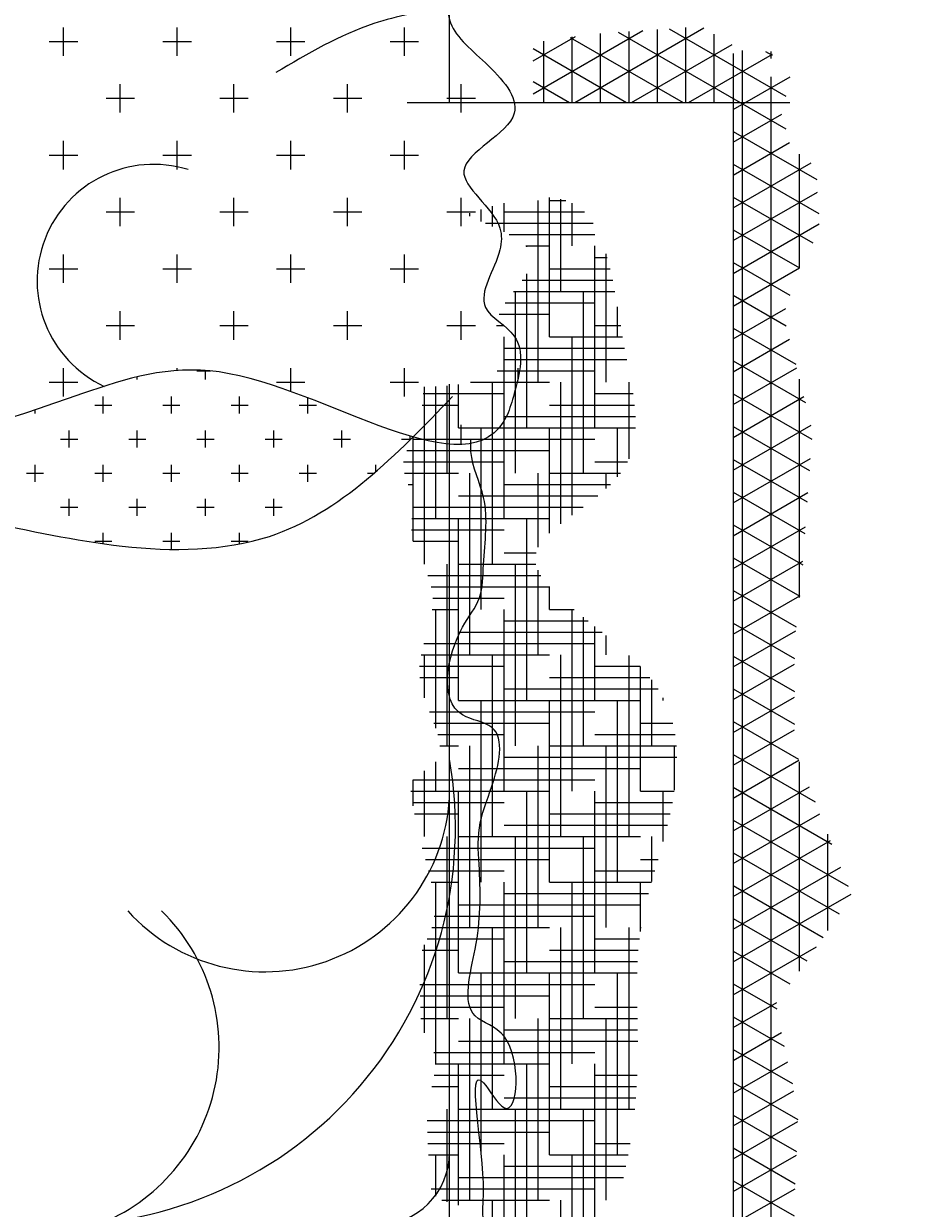
# Model space of a CAD drawing. Units: inches. Extents: x 2330 to 3943, y 1763 to 3461.
# Tile 18 of 40: x 3179 to 3231, y 2593 to 2662. Entities that reach past the tile are written whole.
import ezdxf

# ---------------------------------------------------------------- set-up
doc = ezdxf.new("R2010")
doc.units = ezdxf.units.IN
doc.layers.add('A-ANNO-DIMS', color=2, linetype='Continuous', lineweight=18)
doc.layers.add('A-FURN', color=8, linetype='Continuous', lineweight=13)
doc.styles.get("Standard").update_dxf_attribs({"font": 'arial.ttf'})
doc.dimstyles.get("Standard").update_dxf_attribs({"dimtxt": 0.18, "dimasz": 0.18, "dimexe": 0.18, "dimexo": 0.0625, "dimgap": 0.09, "dimtad": 0, "dimtih": 1, "dimtoh": 1, "dimdec": 4, "dimzin": 0, "dimdsep": 46, "dimtxsty": 'Standard', "dimcen": 0.09, "dimadec": 0, "dimazin": 0, "dimtfac": 1, "dimtdec": 4, "dimtofl": 0, "dimtmove": 0, "dimatfit": 3, "dimfxl": 1, "dimtolj": 1, "dimtzin": 0, "dimarcsym": 0})

# ---------------------------------------------------------------- blocks, each defined once
blk = doc.blocks.new('A$C200C7901')
for p, q in [((2, 1.6055), (2, 2.3334)), ((2.3121, 1.6596), (2.3121, 0.0201)), ((1.9533, 1.6055), (2.3741, 1.6055)), ((1.9533, 1.6055), (2.3741, 1.6055)), ((2, 0.2957), (2, 1.2957)), ((2.0224, 0.9977), (2.0224, 1.1977)), ((2.0224, 0.9977), (2.0224, 1.1977)), ((1.9974, 0.5977), (1.9974, 0.7977)), ((1.9974, 0.5977), (1.9974, 0.7977)), ((2.0724, 0.5977), (2.0724, 0.7977)), ((2.0724, 0.5977), (2.0724, 0.7977)), ((2.1474, 0.5977), (2.1474, 0.7977)), ((2.1474, 0.5977), (2.1474, 0.7977)), ((1.9849, 0.5477), (1.9849, 0.7477)), ((1.9849, 0.5477), (1.9849, 0.7477)), ((2.0599, 0.5477), (2.0599, 0.7477)), ((2.0599, 0.5477), (2.0599, 0.7477)), ((2.1349, 0.5477), (2.1349, 0.7477)), ((2.1349, 0.5477), (2.1349, 0.7477))]:
    blk.add_line(p, q)
at = {"linetype": 'ByBlock'}
for p, q in [((1.5754, 1.657), (1.5754, 1.6883)), ((1.5754, 1.657), (1.5754, 1.6883)), ((1.7004, 1.657), (1.7004, 1.6883)), ((1.7004, 1.657), (1.7004, 1.6883)), ((1.8254, 1.657), (1.8254, 1.6883)), ((1.8254, 1.657), (1.8254, 1.6883)), ((1.9504, 1.657), (1.9504, 1.6883)), ((1.9504, 1.657), (1.9504, 1.6883)), ((2.0919, 1.6152), (2.2125, 1.6848)), ((2.0919, 1.6152), (2.2125, 1.6848)), ((2.1377, 1.6055), (2.2798, 1.6876)), ((2.1377, 1.6055), (2.2798, 1.6876)), ((2.1662, 1.6055), (2.1662, 1.6817)), ((2.1662, 1.6055), (2.1662, 1.6817)), ((2.1854, 1.683), (2.3697, 1.5766)), ((2.1854, 1.683), (2.3697, 1.5766)), ((2.1974, 1.6055), (2.1974, 1.6838)), ((2.1974, 1.6055), (2.1974, 1.6838)), ((2.2287, 1.6055), (2.2287, 1.6859)), ((2.2287, 1.6055), (2.2287, 1.6859)), ((2.2414, 1.6868), (2.3699, 1.6126)), ((2.2414, 1.6868), (2.3699, 1.6126)), ((2.2599, 1.6055), (2.2599, 1.688)), ((2.2599, 1.6055), (2.2599, 1.688)), ((1.5597, 1.6727), (1.591, 1.6727)), ((1.5597, 1.6727), (1.591, 1.6727)), ((1.6847, 1.6727), (1.716, 1.6727)), ((1.6847, 1.6727), (1.716, 1.6727)), ((1.8097, 1.6727), (1.841, 1.6727)), ((1.8097, 1.6727), (1.841, 1.6727)), ((1.9347, 1.6727), (1.966, 1.6727)), ((1.9347, 1.6727), (1.966, 1.6727)), ((2.0919, 1.6513), (2.1386, 1.6782)), ((2.0919, 1.6513), (2.1386, 1.6782)), ((2.1037, 1.6055), (2.1037, 1.673)), ((2.1037, 1.6055), (2.1037, 1.673)), ((2.1327, 1.6773), (2.2571, 1.6055)), ((2.1327, 1.6773), (2.2571, 1.6055)), ((2.1349, 1.6055), (2.1349, 1.6777)), ((2.1349, 1.6055), (2.1349, 1.6777)), ((2.2002, 1.6055), (2.3109, 1.6694)), ((2.2002, 1.6055), (2.3109, 1.6694)), ((2.2912, 1.6055), (2.2912, 1.6809)), ((2.2912, 1.6055), (2.2912, 1.6809)), ((2.0919, 1.6649), (2.1946, 1.6055)), ((2.0919, 1.6649), (2.1946, 1.6055)), ((2.2627, 1.6055), (2.3551, 1.6589)), ((2.2627, 1.6055), (2.3551, 1.6589)), ((2.3224, 0.0468), (2.3224, 1.6627)), ((2.3224, 0.0468), (2.3224, 1.6627)), ((2.3476, 1.6616), (2.3547, 1.6575)), ((2.3476, 1.6616), (2.3547, 1.6575)), ((2.3537, 1.6539), (2.3537, 1.6616)), ((2.3537, 1.6539), (2.3537, 1.6616)), ((2.3121, 1.598), (2.3745, 1.634)), ((2.3121, 1.598), (2.3745, 1.634)), ((2.3537, 0.0056), (2.3537, 1.634)), ((2.3537, 0.0056), (2.3537, 1.634)), ((1.6379, 1.5945), (1.6379, 1.6258)), ((1.6379, 1.5945), (1.6379, 1.6258)), ((1.7629, 1.5945), (1.7629, 1.6258)), ((1.7629, 1.5945), (1.7629, 1.6258)), ((1.8879, 1.5945), (1.8879, 1.6258)), ((1.8879, 1.5945), (1.8879, 1.6258)), ((2.0129, 1.5945), (2.0129, 1.6258)), ((2.0129, 1.5945), (2.0129, 1.6258)), ((2.0919, 1.6288), (2.1321, 1.6055)), ((2.0919, 1.6288), (2.1321, 1.6055)), ((1.6222, 1.6102), (1.6535, 1.6102)), ((1.6222, 1.6102), (1.6535, 1.6102)), ((1.7472, 1.6102), (1.7785, 1.6102)), ((1.7472, 1.6102), (1.7785, 1.6102)), ((1.8722, 1.6102), (1.9035, 1.6102)), ((1.8722, 1.6102), (1.9035, 1.6102)), ((1.9972, 1.6102), (2.0285, 1.6102)), ((1.9972, 1.6102), (2.0285, 1.6102)), ((2.3121, 1.5619), (2.3654, 1.5926)), ((2.3121, 1.5619), (2.3654, 1.5926)), ((2.3121, 1.5738), (2.404, 1.5208)), ((2.3121, 1.5738), (2.404, 1.5208)), ((1.5754, 1.532), (1.5754, 1.5633)), ((1.5754, 1.532), (1.5754, 1.5633)), ((1.7004, 1.532), (1.7004, 1.5633)), ((1.7004, 1.532), (1.7004, 1.5633)), ((1.8254, 1.532), (1.8254, 1.5633)), ((1.8254, 1.532), (1.8254, 1.5633)), ((1.9504, 1.532), (1.9504, 1.5633)), ((1.9504, 1.532), (1.9504, 1.5633)), ((2.3121, 1.5258), (2.3739, 1.5615)), ((2.3121, 1.5258), (2.3739, 1.5615)), ((1.5597, 1.5477), (1.591, 1.5477)), ((1.5597, 1.5477), (1.591, 1.5477)), ((1.6847, 1.5477), (1.716, 1.5477)), ((1.6847, 1.5477), (1.716, 1.5477)), ((1.8097, 1.5477), (1.841, 1.5477)), ((1.8097, 1.5477), (1.841, 1.5477)), ((1.9347, 1.5477), (1.966, 1.5477)), ((1.9347, 1.5477), (1.966, 1.5477)), ((2.3121, 1.4897), (2.3979, 1.5393)), ((2.3121, 1.4897), (2.3979, 1.5393)), ((2.3849, 1.4236), (2.3849, 1.5486)), ((2.3849, 1.4236), (2.3849, 1.5486)), ((2.3121, 1.5377), (2.406, 1.4835)), ((2.3121, 1.5377), (2.406, 1.4835)), ((1.6379, 1.4695), (1.6379, 1.5008)), ((1.6379, 1.4695), (1.6379, 1.5008)), ((1.7629, 1.4695), (1.7629, 1.5008)), ((1.7629, 1.4695), (1.7629, 1.5008)), ((1.8879, 1.4695), (1.8879, 1.5008)), ((1.8879, 1.4695), (1.8879, 1.5008)), ((2.0129, 1.4695), (2.0129, 1.5008)), ((2.0129, 1.4695), (2.0129, 1.5008)), ((2.1099, 1.3477), (2.1099, 1.5009)), ((2.1099, 1.3477), (2.1099, 1.5009)), ((2.1224, 1.3977), (2.1224, 1.4992)), ((2.1224, 1.3977), (2.1224, 1.4992)), ((2.3121, 1.4537), (2.4047, 1.5071)), ((2.3121, 1.4537), (2.4047, 1.5071)), ((2.3121, 1.5016), (2.3997, 1.4511)), ((2.3121, 1.5016), (2.3997, 1.4511)), ((2.0349, 1.4748), (2.0349, 1.4879)), ((2.0349, 1.4748), (2.0349, 1.4879)), ((2.0474, 1.4691), (2.0474, 1.4915)), ((2.0474, 1.4691), (2.0474, 1.4915)), ((2.0599, 1.4631), (2.0599, 1.4948)), ((2.0599, 1.4631), (2.0599, 1.4948)), ((2.0974, 1.2977), (2.0974, 1.4977)), ((2.0974, 1.2977), (2.0974, 1.4977)), ((2.1099, 1.4977), (2.1279, 1.4977)), ((2.1099, 1.4977), (2.1279, 1.4977)), ((2.1349, 1.4477), (2.1349, 1.4949)), ((2.1349, 1.4477), (2.1349, 1.4949)), ((1.6222, 1.4852), (1.6535, 1.4852)), ((1.6222, 1.4852), (1.6535, 1.4852)), ((1.7472, 1.4852), (1.7785, 1.4852)), ((1.7472, 1.4852), (1.7785, 1.4852)), ((1.8722, 1.4852), (1.9035, 1.4852)), ((1.8722, 1.4852), (1.9035, 1.4852)), ((1.9972, 1.4852), (2.0285, 1.4852)), ((1.9972, 1.4852), (2.0285, 1.4852)), ((2.0224, 1.4805), (2.0224, 1.4839)), ((2.0224, 1.4805), (2.0224, 1.4839)), ((2.0599, 1.4852), (2.1484, 1.4852)), ((2.0599, 1.4852), (2.1484, 1.4852)), ((2.0397, 1.4727), (2.1581, 1.4727)), ((2.0397, 1.4727), (2.1581, 1.4727)), ((2.0656, 1.4602), (2.1599, 1.4602)), ((2.0656, 1.4602), (2.1599, 1.4602)), ((2.3121, 1.4176), (2.4067, 1.4721)), ((2.3121, 1.4176), (2.4067, 1.4721)), ((2.3121, 1.4655), (2.3849, 1.4235)), ((2.3121, 1.4655), (2.3849, 1.4235)), ((2.084, 1.4477), (2.1099, 1.4477)), ((2.084, 1.4477), (2.1099, 1.4477)), ((2.0849, 1.4468), (2.0849, 1.4477)), ((2.0849, 1.4468), (2.0849, 1.4477)), ((2.1599, 1.2477), (2.1599, 1.4477)), ((2.1599, 1.2477), (2.1599, 1.4477)), ((1.5754, 1.407), (1.5754, 1.4383)), ((1.5754, 1.407), (1.5754, 1.4383)), ((1.7004, 1.407), (1.7004, 1.4383)), ((1.7004, 1.407), (1.7004, 1.4383)), ((1.8254, 1.407), (1.8254, 1.4383)), ((1.8254, 1.407), (1.8254, 1.4383)), ((1.9504, 1.407), (1.9504, 1.4383)), ((1.9504, 1.407), (1.9504, 1.4383)), ((2.1599, 1.4352), (2.1735, 1.4352)), ((2.1599, 1.4352), (2.1735, 1.4352)), ((2.1724, 1.2977), (2.1724, 1.439)), ((2.1724, 1.2977), (2.1724, 1.439)), ((1.5597, 1.4227), (1.591, 1.4227)), ((1.5597, 1.4227), (1.591, 1.4227)), ((1.6847, 1.4227), (1.716, 1.4227)), ((1.6847, 1.4227), (1.716, 1.4227)), ((1.8097, 1.4227), (1.841, 1.4227)), ((1.8097, 1.4227), (1.841, 1.4227)), ((1.9347, 1.4227), (1.966, 1.4227)), ((1.9347, 1.4227), (1.966, 1.4227)), ((2.1099, 1.4227), (2.1767, 1.4227)), ((2.1099, 1.4227), (2.1767, 1.4227)), ((2.3121, 1.4294), (2.3741, 1.3937)), ((2.3121, 1.4294), (2.3741, 1.3937)), ((2.3121, 1.3815), (2.3848, 1.4235)), ((2.3121, 1.3815), (2.3848, 1.4235)), ((2.08, 1.4102), (2.1795, 1.4102)), ((2.08, 1.4102), (2.1795, 1.4102)), ((2.0849, 1.2477), (2.0849, 1.4171)), ((2.0849, 1.2477), (2.0849, 1.4171)), ((2.0703, 1.3977), (2.1819, 1.3977)), ((2.0703, 1.3977), (2.1819, 1.3977)), ((2.0724, 1.1977), (2.0724, 1.3977)), ((2.0724, 1.1977), (2.0724, 1.3977)), ((2.1474, 1.1977), (2.1474, 1.3977)), ((2.1474, 1.1977), (2.1474, 1.3977)), ((2.0612, 1.3852), (2.1599, 1.3852)), ((2.0612, 1.3852), (2.1599, 1.3852)), ((2.3121, 1.3934), (2.3703, 1.3598)), ((2.3121, 1.3934), (2.3703, 1.3598)), ((1.6379, 1.3445), (1.6379, 1.3758)), ((1.6379, 1.3445), (1.6379, 1.3758)), ((1.7629, 1.3445), (1.7629, 1.3758)), ((1.7629, 1.3445), (1.7629, 1.3758)), ((1.8879, 1.3445), (1.8879, 1.3758)), ((1.8879, 1.3445), (1.8879, 1.3758)), ((2.0129, 1.3445), (2.0129, 1.3758)), ((2.0129, 1.3445), (2.0129, 1.3758)), ((2.0545, 1.3727), (2.1099, 1.3727)), ((2.0545, 1.3727), (2.1099, 1.3727)), ((2.1849, 1.3477), (2.1849, 1.3808)), ((2.1849, 1.3477), (2.1849, 1.3808)), ((2.3121, 1.3454), (2.37, 1.3788)), ((2.3121, 1.3454), (2.37, 1.3788)), ((1.6222, 1.3602), (1.6535, 1.3602)), ((1.6222, 1.3602), (1.6535, 1.3602)), ((1.7472, 1.3602), (1.7785, 1.3602)), ((1.7472, 1.3602), (1.7785, 1.3602)), ((1.8722, 1.3602), (1.9035, 1.3602)), ((1.8722, 1.3602), (1.9035, 1.3602)), ((1.9972, 1.3602), (2.0285, 1.3602)), ((1.9972, 1.3602), (2.0285, 1.3602)), ((2.0515, 1.3602), (2.0599, 1.3602)), ((2.0515, 1.3602), (2.0599, 1.3602)), ((2.1599, 1.3602), (2.1883, 1.3602)), ((2.1599, 1.3602), (2.1883, 1.3602)), ((2.3121, 1.3573), (2.3808, 1.3176)), ((2.3121, 1.3573), (2.3808, 1.3176)), ((2.0599, 1.1477), (2.0599, 1.3477)), ((2.0599, 1.1477), (2.0599, 1.3477)), ((2.1099, 1.3477), (2.1904, 1.3477)), ((2.1099, 1.3477), (2.1904, 1.3477)), ((2.1349, 1.1515), (2.1349, 1.3477)), ((2.1349, 1.1515), (2.1349, 1.3477)), ((2.3121, 1.3093), (2.374, 1.345)), ((2.3121, 1.3093), (2.374, 1.345)), ((2.0599, 1.3352), (2.1926, 1.3352)), ((2.0599, 1.3352), (2.1926, 1.3352)), ((2.0594, 1.3227), (2.195, 1.3227)), ((2.0594, 1.3227), (2.195, 1.3227)), ((2.3121, 1.3212), (2.3914, 1.2754)), ((2.3121, 1.3212), (2.3914, 1.2754)), ((1.5754, 1.282), (1.5754, 1.3133)), ((1.5754, 1.282), (1.5754, 1.3133)), ((1.6566, 1.3008), (1.6566, 1.3036)), ((1.6566, 1.3008), (1.6566, 1.3036)), ((1.7004, 1.3106), (1.7004, 1.3133)), ((1.7004, 1.3106), (1.7004, 1.3133)), ((1.7222, 1.3102), (1.7369, 1.3102)), ((1.7222, 1.3102), (1.7369, 1.3102)), ((1.7316, 1.3008), (1.7316, 1.3106)), ((1.7316, 1.3008), (1.7316, 1.3106)), ((1.8254, 1.2876), (1.8254, 1.3133)), ((1.8254, 1.2876), (1.8254, 1.3133)), ((1.9504, 1.282), (1.9504, 1.3133)), ((1.9504, 1.282), (1.9504, 1.3133)), ((2.0524, 1.3102), (2.1599, 1.3102)), ((2.0524, 1.3102), (2.1599, 1.3102)), ((2.0754, 1.3017), (2.0754, 1.3133)), ((2.0754, 1.3017), (2.0754, 1.3133)), ((2.3121, 1.2732), (2.3819, 1.3135)), ((2.3121, 1.2732), (2.3819, 1.3135)), ((1.5597, 1.2977), (1.591, 1.2977)), ((1.5597, 1.2977), (1.591, 1.2977)), ((1.8097, 1.2977), (1.841, 1.2977)), ((1.8097, 1.2977), (1.841, 1.2977)), ((1.9347, 1.2977), (1.966, 1.2977)), ((1.9347, 1.2977), (1.966, 1.2977)), ((1.9724, 1.0977), (1.9724, 1.2927)), ((1.9724, 1.0977), (1.9724, 1.2927)), ((1.9849, 1.1477), (1.9849, 1.293)), ((1.9849, 1.1477), (1.9849, 1.293)), ((1.9974, 1.1977), (1.9974, 1.2939)), ((1.9974, 1.1977), (1.9974, 1.2939)), ((2.0099, 1.2477), (2.0099, 1.2953)), ((2.0099, 1.2477), (2.0099, 1.2953)), ((2.023, 1.2977), (2.1099, 1.2977)), ((2.023, 1.2977), (2.1099, 1.2977)), ((2.0474, 1.0977), (2.0474, 1.2977)), ((2.0474, 1.0977), (2.0474, 1.2977)), ((2.0597, 1.2977), (2.0744, 1.2977)), ((2.0597, 1.2977), (2.0744, 1.2977)), ((2.1224, 1.1421), (2.1224, 1.2977)), ((2.1224, 1.1421), (2.1224, 1.2977)), ((2.1974, 1.2135), (2.1974, 1.2977)), ((2.1974, 1.2135), (2.1974, 1.2977)), ((2.3849, 1.0607), (2.3849, 1.3013)), ((2.3849, 1.0607), (2.3849, 1.3013)), ((1.6191, 1.2633), (1.6191, 1.282)), ((1.6191, 1.2633), (1.6191, 1.282)), ((1.6941, 1.2633), (1.6941, 1.282)), ((1.6941, 1.2633), (1.6941, 1.282)), ((1.7691, 1.2633), (1.7691, 1.282)), ((1.7691, 1.2633), (1.7691, 1.282)), ((1.8441, 1.2633), (1.8441, 1.2806)), ((1.8441, 1.2633), (1.8441, 1.2806)), ((1.9711, 1.2852), (2.0599, 1.2852)), ((1.9711, 1.2852), (2.0599, 1.2852)), ((2.1599, 1.2852), (2.2018, 1.2852)), ((2.1599, 1.2852), (2.2018, 1.2852)), ((2.3121, 1.2851), (2.3985, 1.2352)), ((2.3121, 1.2851), (2.3985, 1.2352)), ((2.3121, 1.2371), (2.3898, 1.282)), ((2.3121, 1.2371), (2.3898, 1.282)), ((1.5441, 1.2633), (1.5441, 1.2675)), ((1.5441, 1.2633), (1.5441, 1.2675)), ((1.6097, 1.2727), (1.6285, 1.2727)), ((1.6097, 1.2727), (1.6285, 1.2727)), ((1.6847, 1.2727), (1.7035, 1.2727)), ((1.6847, 1.2727), (1.7035, 1.2727)), ((1.7597, 1.2727), (1.7785, 1.2727)), ((1.7597, 1.2727), (1.7785, 1.2727)), ((1.8347, 1.2727), (1.8535, 1.2727)), ((1.8347, 1.2727), (1.8535, 1.2727)), ((1.97, 1.2727), (2.0099, 1.2727)), ((1.97, 1.2727), (2.0099, 1.2727)), ((2.1099, 1.2727), (2.2034, 1.2727)), ((2.1099, 1.2727), (2.2034, 1.2727)), ((2.0599, 1.2602), (2.2044, 1.2602)), ((2.0599, 1.2602), (2.2044, 1.2602)), ((1.5816, 1.2258), (1.5816, 1.2445)), ((1.5816, 1.2258), (1.5816, 1.2445)), ((1.6566, 1.2258), (1.6566, 1.2445)), ((1.6566, 1.2258), (1.6566, 1.2445)), ((1.7316, 1.2258), (1.7316, 1.2445)), ((1.7316, 1.2258), (1.7316, 1.2445)), ((1.8066, 1.2258), (1.8066, 1.2445)), ((1.8066, 1.2258), (1.8066, 1.2445)), ((1.8816, 1.2258), (1.8816, 1.2445)), ((1.8816, 1.2258), (1.8816, 1.2445)), ((1.9566, 1.2344), (1.9566, 1.2385)), ((1.9566, 1.2344), (1.9566, 1.2385)), ((2.0099, 1.2477), (2.2045, 1.2477)), ((2.0099, 1.2477), (2.2045, 1.2477)), ((2.0129, 1.2293), (2.0129, 1.2508)), ((2.0129, 1.2293), (2.0129, 1.2508)), ((2.0349, 1.0477), (2.0349, 1.2477)), ((2.0349, 1.0477), (2.0349, 1.2477)), ((2.1099, 1.1315), (2.1099, 1.2477)), ((2.1099, 1.1315), (2.1099, 1.2477)), ((2.1849, 1.1935), (2.1849, 1.2477)), ((2.1849, 1.1935), (2.1849, 1.2477)), ((2.3121, 1.2011), (2.3976, 1.2504)), ((2.3121, 1.2011), (2.3976, 1.2504)), ((2.3121, 1.249), (2.396, 1.2006)), ((2.3121, 1.249), (2.396, 1.2006)), ((1.5722, 1.2352), (1.591, 1.2352)), ((1.5722, 1.2352), (1.591, 1.2352)), ((1.6472, 1.2352), (1.666, 1.2352)), ((1.6472, 1.2352), (1.666, 1.2352)), ((1.7222, 1.2352), (1.741, 1.2352)), ((1.7222, 1.2352), (1.741, 1.2352)), ((1.7972, 1.2352), (1.816, 1.2352)), ((1.7972, 1.2352), (1.816, 1.2352)), ((1.8722, 1.2352), (1.891, 1.2352)), ((1.8722, 1.2352), (1.891, 1.2352)), ((1.9472, 1.2352), (1.9574, 1.2352)), ((1.9472, 1.2352), (1.9574, 1.2352)), ((1.9599, 1.1228), (1.9599, 1.2373)), ((1.9599, 1.1228), (1.9599, 1.2373)), ((1.9599, 1.2352), (2.1599, 1.2352)), ((1.9599, 1.2352), (2.1599, 1.2352)), ((2, 1.2352), (2.0285, 1.2352)), ((2, 1.2352), (2.0285, 1.2352)), ((1.953, 1.2227), (2.1099, 1.2227)), ((1.953, 1.2227), (2.1099, 1.2227)), ((2.3121, 1.165), (2.397, 1.214)), ((2.3121, 1.165), (2.397, 1.214)), ((2.3121, 1.2129), (2.3935, 1.166)), ((2.3121, 1.2129), (2.3935, 1.166)), ((1.5441, 1.1883), (1.5441, 1.207)), ((1.5441, 1.1883), (1.5441, 1.207)), ((1.6191, 1.1883), (1.6191, 1.207)), ((1.6191, 1.1883), (1.6191, 1.207)), ((1.6941, 1.1883), (1.6941, 1.207)), ((1.6941, 1.1883), (1.6941, 1.207)), ((1.7691, 1.1883), (1.7691, 1.207)), ((1.7691, 1.1883), (1.7691, 1.207)), ((1.8441, 1.1883), (1.8441, 1.207)), ((1.8441, 1.1883), (1.8441, 1.207)), ((1.9191, 1.1995), (1.9191, 1.207)), ((1.9191, 1.1995), (1.9191, 1.207)), ((1.9495, 1.2102), (2.0599, 1.2102)), ((1.9495, 1.2102), (2.0599, 1.2102)), ((2.1599, 1.2102), (2.1959, 1.2102)), ((2.1599, 1.2102), (2.1959, 1.2102)), ((1.5347, 1.1977), (1.5535, 1.1977)), ((1.5347, 1.1977), (1.5535, 1.1977)), ((1.6097, 1.1977), (1.6285, 1.1977)), ((1.6097, 1.1977), (1.6285, 1.1977)), ((1.6847, 1.1977), (1.7035, 1.1977)), ((1.6847, 1.1977), (1.7035, 1.1977)), ((1.7597, 1.1977), (1.7785, 1.1977)), ((1.7597, 1.1977), (1.7785, 1.1977)), ((1.8347, 1.1977), (1.8535, 1.1977)), ((1.8347, 1.1977), (1.8535, 1.1977)), ((1.9097, 1.1977), (1.917, 1.1977)), ((1.9097, 1.1977), (1.917, 1.1977)), ((1.9506, 1.1977), (2.0099, 1.1977)), ((1.9506, 1.1977), (2.0099, 1.1977)), ((2.0974, 1.1161), (2.0974, 1.1977)), ((2.0974, 1.1161), (2.0974, 1.1977)), ((2.1099, 1.1977), (2.1882, 1.1977)), ((2.1099, 1.1977), (2.1882, 1.1977)), ((2.1724, 1.1807), (2.1724, 1.1977)), ((2.1724, 1.1807), (2.1724, 1.1977)), ((1.9545, 1.1852), (1.9599, 1.1852)), ((1.9545, 1.1852), (1.9599, 1.1852)), ((2.0599, 1.1852), (2.1772, 1.1852)), ((2.0599, 1.1852), (2.1772, 1.1852)), ((2.3121, 1.1768), (2.3909, 1.1314)), ((2.3121, 1.1768), (2.3909, 1.1314)), ((2.3121, 1.1289), (2.3942, 1.1763)), ((2.3121, 1.1289), (2.3942, 1.1763)), ((1.5816, 1.1508), (1.5816, 1.1695)), ((1.5816, 1.1508), (1.5816, 1.1695)), ((1.6566, 1.1508), (1.6566, 1.1695)), ((1.6566, 1.1508), (1.6566, 1.1695)), ((1.7316, 1.1508), (1.7316, 1.1695)), ((1.7316, 1.1508), (1.7316, 1.1695)), ((1.8066, 1.1508), (1.8066, 1.1695)), ((1.8066, 1.1508), (1.8066, 1.1695)), ((2.0099, 1.1727), (2.1631, 1.1727)), ((2.0099, 1.1727), (2.1631, 1.1727)), ((1.5722, 1.1602), (1.591, 1.1602)), ((1.5722, 1.1602), (1.591, 1.1602)), ((1.6472, 1.1602), (1.666, 1.1602)), ((1.6472, 1.1602), (1.666, 1.1602)), ((1.7222, 1.1602), (1.741, 1.1602)), ((1.7222, 1.1602), (1.741, 1.1602)), ((1.7972, 1.1602), (1.816, 1.1602)), ((1.7972, 1.1602), (1.816, 1.1602)), ((1.9585, 1.1477), (2.1099, 1.1477)), ((1.9585, 1.1477), (2.1099, 1.1477)), ((1.9599, 1.1602), (2.1468, 1.1602)), ((1.9599, 1.1602), (2.1468, 1.1602)), ((2.0099, 0.9477), (2.0099, 1.1477)), ((2.0099, 0.9477), (2.0099, 1.1477)), ((2.0849, 0.9477), (2.0849, 1.1477)), ((2.0849, 0.9477), (2.0849, 1.1477)), ((1.9581, 1.1352), (2.0599, 1.1352)), ((1.9581, 1.1352), (2.0599, 1.1352)), ((2.3121, 1.1408), (2.3884, 1.0967)), ((2.3121, 1.1408), (2.3884, 1.0967)), ((2.3121, 1.0928), (2.3915, 1.1386)), ((2.3121, 1.0928), (2.3915, 1.1386)), ((1.6097, 1.1227), (1.6285, 1.1227)), ((1.6097, 1.1227), (1.6285, 1.1227)), ((1.6191, 1.1201), (1.6191, 1.132)), ((1.6191, 1.1201), (1.6191, 1.132)), ((1.6847, 1.1227), (1.7035, 1.1227)), ((1.6847, 1.1227), (1.7035, 1.1227)), ((1.6941, 1.1139), (1.6941, 1.132)), ((1.6941, 1.1139), (1.6941, 1.132)), ((1.7597, 1.1227), (1.7785, 1.1227)), ((1.7597, 1.1227), (1.7785, 1.1227)), ((1.7691, 1.1198), (1.7691, 1.132)), ((1.7691, 1.1198), (1.7691, 1.132)), ((1.9599, 1.1227), (2.0099, 1.1227)), ((1.9599, 1.1227), (2.0099, 1.1227)), ((2.0599, 1.1102), (2.0951, 1.1102)), ((2.0599, 1.1102), (2.0951, 1.1102)), ((1.9974, 0.8977), (1.9974, 1.0977)), ((1.9974, 0.8977), (1.9974, 1.0977)), ((2.0099, 1.0977), (2.095, 1.0977)), ((2.0099, 1.0977), (2.095, 1.0977)), ((2.0724, 0.8977), (2.0724, 1.0977)), ((2.0724, 0.8977), (2.0724, 1.0977)), ((2.3121, 1.1047), (2.3851, 1.0625)), ((2.3121, 1.1047), (2.3851, 1.0625)), ((2.3121, 1.0567), (2.3887, 1.1009)), ((2.3121, 1.0567), (2.3887, 1.1009)), ((1.9763, 1.0852), (2.1005, 1.0852)), ((1.9763, 1.0852), (2.1005, 1.0852)), ((2.0974, 0.9977), (2.0974, 1.0909)), ((2.0974, 0.9977), (2.0974, 1.0909)), ((1.9799, 1.0727), (2.1099, 1.0727)), ((1.9799, 1.0727), (2.1099, 1.0727)), ((2.1099, 1.0477), (2.1099, 1.0729)), ((2.1099, 1.0477), (2.1099, 1.0729)), ((1.9815, 1.0602), (2.0599, 1.0602)), ((1.9815, 1.0602), (2.0599, 1.0602)), ((2.3121, 1.0686), (2.3813, 1.0286)), ((2.3121, 1.0686), (2.3813, 1.0286)), ((2.3121, 1.0206), (2.3851, 1.0628)), ((2.3121, 1.0206), (2.3851, 1.0628)), ((1.981, 1.0477), (2.0099, 1.0477)), ((1.981, 1.0477), (2.0099, 1.0477)), ((1.9849, 0.9171), (1.9849, 1.0477)), ((1.9849, 0.9171), (1.9849, 1.0477)), ((2.0599, 0.8477), (2.0599, 1.0477)), ((2.0599, 0.8477), (2.0599, 1.0477)), ((2.1099, 1.0477), (2.137, 1.0477)), ((2.1099, 1.0477), (2.137, 1.0477)), ((2.1349, 0.8477), (2.1349, 1.0477)), ((2.1349, 0.8477), (2.1349, 1.0477)), ((2.0599, 1.0352), (2.1523, 1.0352)), ((2.0599, 1.0352), (2.1523, 1.0352)), ((2.1474, 0.8977), (2.1474, 1.0391)), ((2.1474, 0.8977), (2.1474, 1.0391)), ((2.3121, 1.0325), (2.3795, 0.9936)), ((2.3121, 1.0325), (2.3795, 0.9936)), ((2.0099, 1.0227), (2.1678, 1.0227)), ((2.0099, 1.0227), (2.1678, 1.0227)), ((2.1599, 0.9477), (2.1599, 1.029)), ((2.1599, 0.9477), (2.1599, 1.029)), ((2.1724, 0.9977), (2.1724, 1.0189)), ((2.1724, 0.9977), (2.1724, 1.0189)), ((2.3121, 0.9846), (2.3809, 1.0242)), ((2.3121, 0.9846), (2.3809, 1.0242)), ((1.9718, 1.0102), (2.1599, 1.0102)), ((1.9718, 1.0102), (2.1599, 1.0102)), ((1.9688, 0.9977), (2.1099, 0.9977)), ((1.9688, 0.9977), (2.1099, 0.9977)), ((1.9724, 0.9504), (1.9724, 0.9977)), ((1.9724, 0.9504), (1.9724, 0.9977)), ((2.0474, 0.7977), (2.0474, 0.9977)), ((2.0474, 0.7977), (2.0474, 0.9977)), ((2.1224, 0.7977), (2.1224, 0.9977)), ((2.1224, 0.7977), (2.1224, 0.9977)), ((2.1974, 0.7977), (2.1974, 0.9972)), ((2.1974, 0.7977), (2.1974, 0.9972)), ((2.3121, 0.9964), (2.3795, 0.9575)), ((2.3121, 0.9964), (2.3795, 0.9575)), ((1.9671, 0.9852), (2.0599, 0.9852)), ((1.9671, 0.9852), (2.0599, 0.9852)), ((2.1599, 0.9852), (2.2095, 0.9852)), ((2.1599, 0.9852), (2.2095, 0.9852)), ((2.2099, 0.8477), (2.2099, 0.9848)), ((2.2099, 0.8477), (2.2099, 0.9848)), ((2.3121, 0.9485), (2.3795, 0.9874)), ((2.3121, 0.9485), (2.3795, 0.9874)), ((1.9672, 0.9727), (2.0099, 0.9727)), ((1.9672, 0.9727), (2.0099, 0.9727)), ((2.1099, 0.9727), (2.2204, 0.9727)), ((2.1099, 0.9727), (2.2204, 0.9727)), ((2.2224, 0.8977), (2.2224, 0.9702)), ((2.2224, 0.8977), (2.2224, 0.9702)), ((2.0599, 0.9602), (2.2294, 0.9602)), ((2.0599, 0.9602), (2.2294, 0.9602)), ((2.3121, 0.9603), (2.3795, 0.9215)), ((2.3121, 0.9603), (2.3795, 0.9215)), ((2.0099, 0.9477), (2.2099, 0.9477)), ((2.0099, 0.9477), (2.2099, 0.9477)), ((2.0349, 0.7477), (2.0349, 0.9477)), ((2.0349, 0.7477), (2.0349, 0.9477)), ((2.1099, 0.7477), (2.1099, 0.9477)), ((2.1099, 0.7477), (2.1099, 0.9477)), ((2.1849, 0.7477), (2.1849, 0.9477)), ((2.1849, 0.7477), (2.1849, 0.9477)), ((2.2349, 0.9477), (2.2349, 0.9506)), ((2.2349, 0.9477), (2.2349, 0.9506)), ((2.3121, 0.9124), (2.3795, 0.9513)), ((2.3121, 0.9124), (2.3795, 0.9513)), ((1.9781, 0.9352), (2.1599, 0.9352)), ((1.9781, 0.9352), (2.1599, 0.9352)), ((1.9829, 0.9227), (2.1099, 0.9227)), ((1.9829, 0.9227), (2.1099, 0.9227)), ((2.2099, 0.9227), (2.2455, 0.9227)), ((2.2099, 0.9227), (2.2455, 0.9227)), ((2.3121, 0.9243), (2.3838, 0.8829)), ((2.3121, 0.9243), (2.3838, 0.8829)), ((2.3121, 0.8763), (2.3795, 0.9152)), ((2.3121, 0.8763), (2.3795, 0.9152)), ((1.9871, 0.9102), (2.0599, 0.9102)), ((1.9871, 0.9102), (2.0599, 0.9102)), ((2.1599, 0.9102), (2.2481, 0.9102)), ((2.1599, 0.9102), (2.2481, 0.9102)), ((1.9894, 0.8977), (2.0099, 0.8977)), ((1.9894, 0.8977), (2.0099, 0.8977)), ((2.0224, 0.6977), (2.0224, 0.8977)), ((2.0224, 0.6977), (2.0224, 0.8977)), ((2.0974, 0.6977), (2.0974, 0.8977)), ((2.0974, 0.6977), (2.0974, 0.8977)), ((2.1099, 0.8977), (2.2496, 0.8977)), ((2.1099, 0.8977), (2.2496, 0.8977)), ((2.1724, 0.6977), (2.1724, 0.8977)), ((2.1724, 0.6977), (2.1724, 0.8977)), ((2.2474, 0.8489), (2.2474, 0.8977)), ((2.2474, 0.8489), (2.2474, 0.8977)), ((2.3121, 0.8882), (2.4022, 0.8362)), ((2.3121, 0.8882), (2.4022, 0.8362)), ((1.9849, 0.8477), (1.9849, 0.88)), ((1.9849, 0.8477), (1.9849, 0.88)), ((2.0599, 0.8852), (2.2501, 0.8852)), ((2.0599, 0.8852), (2.2501, 0.8852)), ((2.3121, 0.8402), (2.3842, 0.8818)), ((2.3121, 0.8402), (2.3842, 0.8818)), ((2.3849, 0.6497), (2.3849, 0.8801)), ((2.3849, 0.6497), (2.3849, 0.8801)), ((1.9599, 0.8317), (1.9599, 0.8604)), ((1.9599, 0.8317), (1.9599, 0.8604)), ((1.9724, 0.7977), (1.9724, 0.8703)), ((1.9724, 0.7977), (1.9724, 0.8703)), ((2.0099, 0.8727), (2.2099, 0.8727)), ((2.0099, 0.8727), (2.2099, 0.8727)), ((1.9574, 0.8477), (2.1099, 0.8477)), ((1.9574, 0.8477), (2.1099, 0.8477)), ((1.9599, 0.8602), (2.1599, 0.8602)), ((1.9599, 0.8602), (2.1599, 0.8602)), ((2.0099, 0.6477), (2.0099, 0.8477)), ((2.0099, 0.6477), (2.0099, 0.8477)), ((2.0849, 0.6477), (2.0849, 0.8477)), ((2.0849, 0.6477), (2.0849, 0.8477)), ((2.1599, 0.6477), (2.1599, 0.8477)), ((2.1599, 0.6477), (2.1599, 0.8477)), ((2.2099, 0.8477), (2.2472, 0.8477)), ((2.2099, 0.8477), (2.2472, 0.8477)), ((2.2349, 0.7923), (2.2349, 0.8477)), ((2.2349, 0.7923), (2.2349, 0.8477)), ((2.3121, 0.8041), (2.3958, 0.8524)), ((2.3121, 0.8041), (2.3958, 0.8524)), ((2.3121, 0.8521), (2.4205, 0.7895)), ((2.3121, 0.8521), (2.4205, 0.7895)), ((1.9593, 0.8352), (2.0599, 0.8352)), ((1.9593, 0.8352), (2.0599, 0.8352)), ((2.1599, 0.8352), (2.2451, 0.8352)), ((2.1599, 0.8352), (2.2451, 0.8352)), ((1.9615, 0.8227), (2.0099, 0.8227)), ((1.9615, 0.8227), (2.0099, 0.8227)), ((2.1099, 0.8227), (2.2425, 0.8227)), ((2.1099, 0.8227), (2.2425, 0.8227)), ((2.3121, 0.7681), (2.4073, 0.823)), ((2.3121, 0.7681), (2.4073, 0.823)), ((2.0599, 0.8102), (2.2396, 0.8102)), ((2.0599, 0.8102), (2.2396, 0.8102)), ((2.3121, 0.816), (2.4384, 0.7431)), ((2.3121, 0.816), (2.4384, 0.7431)), ((2.0099, 0.7977), (2.2099, 0.7977)), ((2.0099, 0.7977), (2.2099, 0.7977)), ((2.2224, 0.7483), (2.2224, 0.7977)), ((2.2224, 0.7483), (2.2224, 0.7977)), ((2.4162, 0.6946), (2.4162, 0.8006)), ((2.4162, 0.6946), (2.4162, 0.8006)), ((1.9699, 0.7852), (2.1599, 0.7852)), ((1.9699, 0.7852), (2.1599, 0.7852)), ((2.3121, 0.732), (2.4189, 0.7936)), ((2.3121, 0.732), (2.4189, 0.7936)), ((1.9734, 0.7727), (2.1099, 0.7727)), ((1.9734, 0.7727), (2.1099, 0.7727)), ((2.2099, 0.7727), (2.2294, 0.7727)), ((2.2099, 0.7727), (2.2294, 0.7727)), ((2.3121, 0.7799), (2.4287, 0.7126)), ((2.3121, 0.7799), (2.4287, 0.7126)), ((1.9767, 0.7602), (2.0599, 0.7602)), ((1.9767, 0.7602), (2.0599, 0.7602)), ((2.1599, 0.7602), (2.2258, 0.7602)), ((2.1599, 0.7602), (2.2258, 0.7602)), ((2.3121, 0.6959), (2.4303, 0.7641)), ((2.3121, 0.6959), (2.4303, 0.7641)), ((1.9797, 0.7477), (2.0099, 0.7477)), ((1.9797, 0.7477), (2.0099, 0.7477)), ((2.1099, 0.7477), (2.2222, 0.7477)), ((2.1099, 0.7477), (2.2222, 0.7477)), ((2.2099, 0.6933), (2.2099, 0.7477)), ((2.2099, 0.6933), (2.2099, 0.7477)), ((2.3121, 0.7438), (2.4108, 0.6869)), ((2.3121, 0.7438), (2.4108, 0.6869)), ((2.0599, 0.7352), (2.2188, 0.7352)), ((2.0599, 0.7352), (2.2188, 0.7352)), ((2.3121, 0.6598), (2.4417, 0.7346)), ((2.3121, 0.6598), (2.4417, 0.7346)), ((2.0099, 0.7227), (2.2099, 0.7227)), ((2.0099, 0.7227), (2.2099, 0.7227)), ((1.9831, 0.7102), (2.1599, 0.7102)), ((1.9831, 0.7102), (2.1599, 0.7102)), ((2.3121, 0.7078), (2.3929, 0.6611)), ((2.3121, 0.7078), (2.3929, 0.6611)), ((1.9804, 0.6977), (2.1099, 0.6977)), ((1.9804, 0.6977), (2.1099, 0.6977)), ((2.0474, 0.4977), (2.0474, 0.6977)), ((2.0474, 0.4977), (2.0474, 0.6977)), ((2.1224, 0.4977), (2.1224, 0.6977)), ((2.1224, 0.4977), (2.1224, 0.6977)), ((2.1974, 0.4977), (2.1974, 0.6977)), ((2.1974, 0.4977), (2.1974, 0.6977)), ((2.2099, 0.6977), (2.2106, 0.6977)), ((2.2099, 0.6977), (2.2106, 0.6977)), ((1.9724, 0.5818), (1.9724, 0.6786)), ((1.9724, 0.5818), (1.9724, 0.6786)), ((1.9753, 0.6852), (2.0599, 0.6852)), ((1.9753, 0.6852), (2.0599, 0.6852)), ((2.1599, 0.6852), (2.2088, 0.6852)), ((2.1599, 0.6852), (2.2088, 0.6852)), ((1.97, 0.6727), (2.0099, 0.6727)), ((1.97, 0.6727), (2.0099, 0.6727)), ((2.1099, 0.6727), (2.2075, 0.6727)), ((2.1099, 0.6727), (2.2075, 0.6727)), ((2.3121, 0.6237), (2.4036, 0.6765)), ((2.3121, 0.6237), (2.4036, 0.6765)), ((2.3121, 0.6717), (2.3744, 0.6357)), ((2.3121, 0.6717), (2.3744, 0.6357)), ((2.0599, 0.6602), (2.2067, 0.6602)), ((2.0599, 0.6602), (2.2067, 0.6602)), ((2.0099, 0.6477), (2.2062, 0.6477)), ((2.0099, 0.6477), (2.2062, 0.6477)), ((2.0349, 0.4477), (2.0349, 0.6477)), ((2.0349, 0.4477), (2.0349, 0.6477)), ((2.1099, 0.4477), (2.1099, 0.6477)), ((2.1099, 0.4477), (2.1099, 0.6477)), ((2.1849, 0.4477), (2.1849, 0.6477)), ((2.1849, 0.4477), (2.1849, 0.6477)), ((1.9673, 0.6352), (2.1599, 0.6352)), ((1.9673, 0.6352), (2.1599, 0.6352)), ((2.3121, 0.6356), (2.3598, 0.6081)), ((2.3121, 0.6356), (2.3598, 0.6081)), ((1.9678, 0.6227), (2.1099, 0.6227)), ((1.9678, 0.6227), (2.1099, 0.6227)), ((2.3121, 0.5876), (2.3598, 0.6151)), ((2.3121, 0.5876), (2.3598, 0.6151)), ((1.9679, 0.6102), (2.0599, 0.6102)), ((1.9679, 0.6102), (2.0599, 0.6102)), ((2.1599, 0.6102), (2.2064, 0.6102)), ((2.1599, 0.6102), (2.2064, 0.6102)), ((1.9685, 0.5977), (2.0099, 0.5977)), ((1.9685, 0.5977), (2.0099, 0.5977)), ((2.0224, 0.3977), (2.0224, 0.5977)), ((2.0224, 0.3977), (2.0224, 0.5977)), ((2.0974, 0.3977), (2.0974, 0.5977)), ((2.0974, 0.3977), (2.0974, 0.5977)), ((2.1099, 0.5977), (2.2066, 0.5977)), ((2.1099, 0.5977), (2.2066, 0.5977)), ((2.1724, 0.3977), (2.1724, 0.5977)), ((2.1724, 0.3977), (2.1724, 0.5977)), ((2.3121, 0.5995), (2.3682, 0.5671)), ((2.3121, 0.5995), (2.3682, 0.5671)), ((2.0599, 0.5852), (2.2069, 0.5852)), ((2.0599, 0.5852), (2.2069, 0.5852)), ((2.3121, 0.5515), (2.365, 0.5821)), ((2.3121, 0.5515), (2.365, 0.5821)), ((2.0099, 0.5727), (2.207, 0.5727)), ((2.0099, 0.5727), (2.207, 0.5727)), ((2.3121, 0.5634), (2.3771, 0.5259)), ((2.3121, 0.5634), (2.3771, 0.5259)), ((1.9827, 0.5602), (2.1599, 0.5602)), ((1.9827, 0.5602), (2.1599, 0.5602)), ((1.9842, 0.5477), (2.1099, 0.5477)), ((1.9842, 0.5477), (2.1099, 0.5477)), ((2.0099, 0.3923), (2.0099, 0.5477)), ((2.0099, 0.3923), (2.0099, 0.5477)), ((2.0849, 0.3477), (2.0849, 0.5477)), ((2.0849, 0.3477), (2.0849, 0.5477)), ((2.1599, 0.3477), (2.1599, 0.5477)), ((2.1599, 0.3477), (2.1599, 0.5477)), ((2.3121, 0.5155), (2.3719, 0.55)), ((2.3121, 0.5155), (2.3719, 0.55)), ((1.9831, 0.5352), (2.0599, 0.5352)), ((1.9831, 0.5352), (2.0599, 0.5352)), ((2.1599, 0.5352), (2.2065, 0.5352)), ((2.1599, 0.5352), (2.2065, 0.5352)), ((1.9807, 0.5227), (2.0099, 0.5227)), ((1.9807, 0.5227), (2.0099, 0.5227)), ((2.1099, 0.5227), (2.2058, 0.5227)), ((2.1099, 0.5227), (2.2058, 0.5227)), ((2.3121, 0.5273), (2.383, 0.4864)), ((2.3121, 0.5273), (2.383, 0.4864)), ((2.0599, 0.5102), (2.2049, 0.5102)), ((2.0599, 0.5102), (2.2049, 0.5102)), ((2.3121, 0.4794), (2.3788, 0.5179)), ((2.3121, 0.4794), (2.3788, 0.5179)), ((1.9974, 0.3957), (1.9974, 0.4977)), ((1.9974, 0.3957), (1.9974, 0.4977)), ((2.0099, 0.4977), (2.2038, 0.4977)), ((2.0099, 0.4977), (2.2038, 0.4977)), ((2.0724, 0.2977), (2.0724, 0.4977)), ((2.0724, 0.2977), (2.0724, 0.4977)), ((2.1474, 0.2977), (2.1474, 0.4977)), ((2.1474, 0.2977), (2.1474, 0.4977)), ((1.9755, 0.4852), (2.1599, 0.4852)), ((1.9755, 0.4852), (2.1599, 0.4852)), ((2.3121, 0.4912), (2.3817, 0.4511)), ((2.3121, 0.4912), (2.3817, 0.4511)), ((2.3121, 0.4433), (2.383, 0.4842)), ((2.3121, 0.4433), (2.383, 0.4842)), ((1.9757, 0.4727), (2.1099, 0.4727)), ((1.9757, 0.4727), (2.1099, 0.4727)), ((1.9762, 0.4602), (2.0599, 0.4602)), ((1.9762, 0.4602), (2.0599, 0.4602)), ((2.1599, 0.4602), (2.1987, 0.4602)), ((2.1599, 0.4602), (2.1987, 0.4602)), ((1.9768, 0.4477), (2.0099, 0.4477)), ((1.9768, 0.4477), (2.0099, 0.4477)), ((1.9849, 0.402), (1.9849, 0.4477)), ((1.9849, 0.402), (1.9849, 0.4477)), ((2.0599, 0.2903), (2.0599, 0.4477)), ((2.0599, 0.2903), (2.0599, 0.4477)), ((2.1099, 0.4477), (2.1965, 0.4477)), ((2.1099, 0.4477), (2.1965, 0.4477)), ((2.1349, 0.2582), (2.1349, 0.4477)), ((2.1349, 0.2582), (2.1349, 0.4477)), ((2.3121, 0.4552), (2.3803, 0.4158)), ((2.3121, 0.4552), (2.3803, 0.4158)), ((2.3121, 0.4072), (2.3815, 0.4473)), ((2.3121, 0.4072), (2.3815, 0.4473)), ((2.0599, 0.4352), (2.194, 0.4352)), ((2.0599, 0.4352), (2.194, 0.4352)), ((2.0099, 0.4227), (2.1913, 0.4227)), ((2.0099, 0.4227), (2.1913, 0.4227)), ((2.3121, 0.4191), (2.3789, 0.3805)), ((2.3121, 0.4191), (2.3789, 0.3805)), ((1.9797, 0.4102), (2.1599, 0.4102)), ((1.9797, 0.4102), (2.1599, 0.4102)), ((2.3121, 0.3711), (2.3801, 0.4103)), ((2.3121, 0.3711), (2.3801, 0.4103)), ((1.9915, 0.3977), (2.1099, 0.3977)), ((1.9915, 0.3977), (2.1099, 0.3977)), ((2.0474, 0.2905), (2.0474, 0.3977)), ((2.0474, 0.2905), (2.0474, 0.3977)), ((2.1224, 0.2385), (2.1224, 0.3977)), ((2.1224, 0.2385), (2.1224, 0.3977))]:
    blk.add_line(p, q, dxfattribs=at)
blk.add_arc((1.6746, 1.4093), 0.1282, 72.7909, 244.8695, dxfattribs=at)
blk.add_arc((1.6746, 1.4093), 0.1282, 72.7909, 244.8695, dxfattribs=at)
for centre, radius, start, end in [((1.5693, 0.8075), 0.4372, 269.0679, 9.9322), ((1.7969, 0.8525), 0.2035, 222.1514, 356.4639), ((1.5372, 0.5659), 0.2094, 290.9415, 45.7647), ((1.92, 0.4503), 0.08, 270, 0)]:
    blk.add_arc(centre, radius, start, end)
for points, knots in [([(0.4485, 1.7835), (0.4321, 1.7496), (0.4062, 1.6964), (0.49, 1.6713), (0.4719, 1.5969), (0.4123, 1.592), (0.4233, 1.5337), (0.4954, 1.5086), (0.4012, 1.4738), (0.3253, 1.4306), (0.4113, 1.3764), (0.3688, 1.3065), (0.5579, 1.2663), (0.741, 1.4533), (1.1127, 1.1109), (1.4811, 1.2478), (1.7885, 1.3492), (2.0357, 1.1637), (2.0748, 1.2974), (2.0876, 1.349), (2.0192, 1.3805), (2.0564, 1.4298), (2.0588, 1.4846), (1.9759, 1.5349), (2.1004, 1.5845), (2.0397, 1.6519), (1.971, 1.7053), (2.1104, 1.8981), (1.5946, 1.7967), (1.2448, 1.7472), (0.8129, 1.7935), (0.4953, 1.8548), (0.4582, 1.7983), (0.4485, 1.7835)], [0, 0, 0, 0, 88.420092, 139.08588, 204.302936, 239.695496, 287.801042, 327.365471, 412.960499, 463.626286, 552.059846, 584.668336, 662.614915, 940.993281, 1309.926334, 1844.022653, 1996.276242, 2316.43048, 2341.441004, 2404.707416, 2449.463774, 2514.680778, 2538.40571, 2613.031547, 2697.13096, 2760.903931, 2822.692699, 2945.47, 3215.060018, 3725.584917, 4361.974444, 4504.671998, 4555.32777, 4555.32777, 4555.32777, 4555.32777]), ([(0.4856, 1.3429), (0.5504, 1.3182), (0.6715, 1.2721), (0.8374, 1.0498), (1.1164, 1.1183), (1.3878, 1.1816), (1.5888, 1.1102), (1.8403, 1.1127), (1.9415, 1.2178), (2.0032, 1.2819)], [0, 0, 0, 0, 205.411753, 383.654933, 772.067458, 921.644661, 1226.793228, 1388.983508, 1642.292305, 1642.292305, 1642.292305, 1642.292305])]:
    blk.add_open_spline(points, degree=3, knots=knots)
for points, knots in [([(1.996, 1.7104), (1.9692, 1.7057), (1.9025, 1.6938), (1.844, 1.6592), (1.809, 1.6385)], [0, 0, 0, 0, 81.132613, 201.738644, 201.738644, 201.738644, 201.738644]), ([(1.996, 1.7104), (1.9692, 1.7057), (1.9025, 1.6938), (1.844, 1.6592), (1.809, 1.6385)], [0, 0, 0, 0, 81.132613, 201.738644, 201.738644, 201.738644, 201.738644]), ([(0.473, 1.2954), (0.4739, 1.2781), (0.4755, 1.2477), (0.5032, 1.2084), (0.4801, 1.1701), (0.4928, 1.1255), (0.4674, 1.0912), (0.4579, 1.0351), (0.501, 0.9724), (0.4311, 0.8832), (0.4902, 0.8637), (0.4843, 0.8288), (0.4774, 0.7906), (0.4625, 0.7457), (0.459, 0.6999), (0.4816, 0.6664), (0.4748, 0.625), (0.4791, 0.5889), (0.4533, 0.5528), (0.4738, 0.5004), (0.4658, 0.4502), (0.4696, 0.3946), (0.4189, 0.3935), (0.4493, 0.3684), (0.4694, 0.3857), (0.4922, 0.3576), (0.5297, 0.3262), (0.5917, 0.3353), (0.6454, 0.3754), (0.7083, 0.3741), (0.7643, 0.3328), (0.826, 0.346), (0.925, 0.3388), (1.0353, 0.3593), (1.1561, 0.3744), (1.2477, 0.3154), (1.3302, 0.3474), (1.4086, 0.3512), (1.5217, 0.3878), (1.6362, 0.3176), (1.7682, 0.3285), (1.8402, 0.3019), (1.9071, 0.3529), (1.9647, 0.3412), (2.0795, 0.2948), (2.0472, 0.3498), (2.0343, 0.3772), (2.0435, 0.43), (2.0109, 0.5782), (2.0746, 0.4643), (2.0805, 0.584), (2.0084, 0.5979), (2.0343, 0.6846), (2.0344, 0.746), (2.0293, 0.8096), (2.0489, 0.8545), (2.0652, 0.9218), (1.9842, 0.9297), (2.0007, 1.0162), (2.0367, 1.0585), (2.0367, 1.1102), (2.0457, 1.1647), (2.0226, 1.2084), (2.0234, 1.2306), (2.0236, 1.2352)], [0, 0, 0, 0, 51.660678, 90.967412, 128.902454, 170.303599, 219.852997, 247.834962, 336.321557, 429.35469, 458.821847, 477.222321, 524.135809, 581.038434, 617.839381, 657.146115, 693.947125, 740.178081, 760.753248, 820.731705, 885.133458, 928.777044, 953.563729, 976.574207, 995.553042, 1018.563482, 1064.584401, 1147.951297, 1174.787598, 1266.851571, 1308.018447, 1377.066427, 1441.511314, 1608.245014, 1714.11869, 1792.771707, 1913.247991, 1954.931389, 2029.864445, 2259.189419, 2305.221512, 2429.507982, 2456.344283, 2543.92595, 2627.925037, 2662.96218, 2687.736879, 2719.937755, 2839.540991, 2875.47895, 2953.681041, 2993.270313, 3066.872333, 3154.395764, 3200.397042, 3248.426375, 3312.828127, 3347.881398, 3444.484026, 3481.577522, 3518.665244, 3592.267265, 3644.719162, 3658.519501, 3658.519501, 3658.519501, 3658.519501])]:
    blk.add_open_spline(points, degree=3, knots=knots, dxfattribs=at)
blk = doc.blocks.new('*D95')
at = {"layer": 'A-ANNO-DIMS', "color": 0, "lineweight": -2, "transparency": 16777216}
for p, q in [((3105.603, 2727.687), (3105.783, 2727.687)), ((3105.693, 2727.597), (3105.693, 2727.777)), ((3606.312, 2659.69), (3418.758, 2685.165))]:
    blk.add_line(p, q, dxfattribs=at)
at = {"layer": 'A-ANNO-DIMS', "color": 0, "transparency": 16777216}
blk.add_solid([(3418.762, 2685.195), (3418.754, 2685.135), (3418.58, 2685.189)], dxfattribs=at)
at = {"layer": 'Defpoints', "color": 0, "transparency": 16777216}
for p in [(3105.693, 2727.687), (3418.58, 2685.189)]:
    blk.add_point(p, dxfattribs=at)
at = {"layer": 'A-ANNO-DIMS', "color": 0, "transparency": 16777216, "insert": (3606.862, 2659.69), "char_height": 0.18, "attachment_point": 5}
blk.add_mtext('\\A1;R315.76', dxfattribs=at)
blk = doc.blocks.new('*D97')
at = {"layer": 'A-ANNO-DIMS', "color": 0, "lineweight": -2, "transparency": 16777216}
for p, q in [((3105.603, 2727.687), (3105.783, 2727.687)), ((3105.693, 2727.597), (3105.693, 2727.777)), ((3589.166, 2615.071), (3408.039, 2657.261))]:
    blk.add_line(p, q, dxfattribs=at)
at = {"layer": 'A-ANNO-DIMS', "color": 0, "transparency": 16777216}
blk.add_solid([(3408.046, 2657.29), (3408.032, 2657.232), (3407.864, 2657.302)], dxfattribs=at)
at = {"layer": 'Defpoints', "color": 0, "transparency": 16777216}
for p in [(3105.693, 2727.687), (3407.864, 2657.302)]:
    blk.add_point(p, dxfattribs=at)
at = {"layer": 'A-ANNO-DIMS', "color": 0, "transparency": 16777216, "insert": (3589.911, 2615.071), "char_height": 0.18, "attachment_point": 5}
blk.add_mtext('\\A1;2X R310.26', dxfattribs=at)
blk = doc.blocks.new('*D98')
at = {"layer": 'A-ANNO-DIMS', "color": 0, "lineweight": -2, "transparency": 16777216}
for p, q in [((3105.603, 2727.687), (3105.783, 2727.687)), ((3105.693, 2727.597), (3105.693, 2727.777)), ((3519.334, 2463.489), (3364.371, 2562.466)), ((3519.514, 2463.489), (3519.334, 2463.489))]:
    blk.add_line(p, q, dxfattribs=at)
at = {"layer": 'A-ANNO-DIMS', "color": 0, "transparency": 16777216}
blk.add_solid([(3364.387, 2562.491), (3364.355, 2562.441), (3364.219, 2562.563)], dxfattribs=at)
at = {"layer": 'Defpoints', "color": 0, "transparency": 16777216}
for p in [(3105.693, 2727.687), (3364.219, 2562.563)]:
    blk.add_point(p, dxfattribs=at)
at = {"layer": 'A-ANNO-DIMS', "color": 0, "transparency": 16777216, "insert": (3520.257, 2463.489), "char_height": 0.18, "attachment_point": 5}
blk.add_mtext('\\A1;3X R306.76', dxfattribs=at)

msp = doc.modelspace()

# ---------------------------------------------------------------- block references
at = {"layer": 'A-FURN', "xscale": 52.5181391560459, "yscale": 52.5181391560459, "zscale": 52.5181391560459}
msp.add_blockref('A$C200C7901', (3098.8053, 2572.8601), dxfattribs=at)

# ---------------------------------------------------------------- dimensions: what is measured, and where the dimension line sits
at = {"layer": 'A-ANNO-DIMS'}
dim = msp.add_radius_dim(center=(3105.6935, 2727.6869), mpoint=(3418.58, 2685.189), dimstyle='Standard', override={"dimdec": 2, "dimlfac": 1, "dimrnd": 0, "dimzin": 0, "dimdsep": 46, "dimlunit": 2}, dxfattribs=at)
dim.commit()
dim.dimension.update_dxf_attribs({"geometry": '*D95', "text_midpoint": (3606.3119, 2659.6902), "dimtype": 164})
for mpoint, text, picture, middle in [((3407.8638, 2657.302), '2X <>', '*D97', (3589.166, 2615.0711)), ((3364.219, 2562.563), '3X <>', '*D98', (3520.2574, 2463.4886))]:
    dim = msp.add_radius_dim(center=(3105.6935, 2727.6869), mpoint=mpoint, text=text, dimstyle='Standard', override={"dimdec": 2, "dimlfac": 1, "dimrnd": 0, "dimzin": 0, "dimdsep": 46, "dimlunit": 2}, dxfattribs=at)
    dim.commit()
    dim.dimension.update_dxf_attribs({"geometry": picture, "text_midpoint": middle, "dimtype": 164})

doc.saveas('drawing.dxf')
